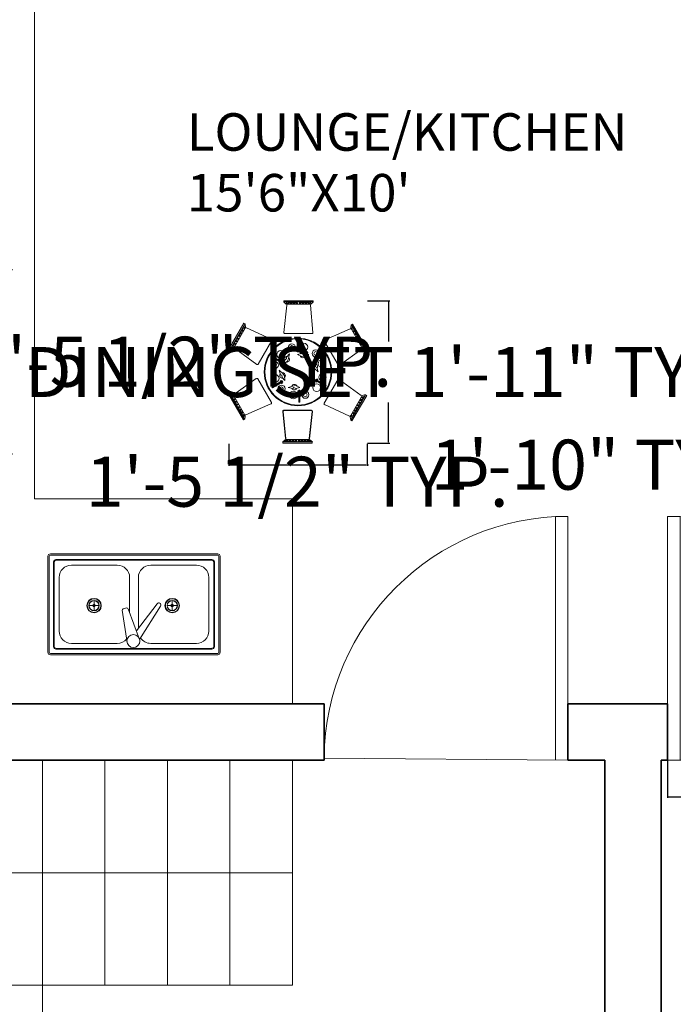
# Model space of a CAD drawing. Units: inches. Extents: x 125 to 976, y 231 to 853.
# Tile 3 of 16: x 219 to 324, y 455 to 613. Entities that reach past the tile are written whole.
import ezdxf

# ---------------------------------------------------------------- set-up
doc = ezdxf.new("R2010")
doc.units = ezdxf.units.IN
doc.header["$MEASUREMENT"] = 0
for name, color, linetype, lineweight in [('A-ANNO-DIMS', 2, 'Continuous', 18), ('A-AREA-IDEN', 7, 'Continuous', 18), ('A-DOOR', 3, 'Continuous', 18), ('A-FLOR-CASE', 32, 'Continuous', 18), ('A-FLOR-FIXT', 9, 'Continuous', 18), ('A-FLOR-STRS', 7, 'Continuous', 18), ('A-WALL', 7, 'Continuous', 35), ('Furniture', 8, 'Continuous', 15)]:
    doc.layers.add(name, color=color, linetype=linetype, lineweight=lineweight)
doc.styles.get("Standard").update_dxf_attribs({"font": 'italic8.shx'})
doc.dimstyles.get("Standard").update_dxf_attribs({"dimtxt": 8, "dimasz": 0.18, "dimexe": 0.18, "dimexo": 0.0625, "dimgap": 0.09, "dimtad": 0, "dimtih": 1, "dimtoh": 1, "dimdec": 4, "dimzin": 0, "dimdsep": 46, "dimlunit": 3, "dimtxsty": 'Standard', "dimcen": 0.09, "dimclrt": 4, "dimadec": 0, "dimazin": 0, "dimtfac": 1, "dimtdec": 4, "dimtofl": 0, "dimtmove": 0, "dimatfit": 3, "dimfxl": 1, "dimtolj": 1, "dimtzin": 0, "dimarcsym": 0})

# ---------------------------------------------------------------- blocks, each defined once
blk = doc.blocks.new('DINING-SET-ROUND-6')
for p, q in [((8.8, 22.58), (9.2, 22.26)), ((8.82, 17.72), (9.3, 22.08)), ((8.83, 22.8), (8.83, 22.6)), ((13.52, 22.8), (8.83, 22.8)), ((8.83, 22.6), (13.52, 22.6)), ((9.19, 22.53), (9.57, 22.55)), ((9.54, 22.27), (9.19, 22.53)), ((9.2, 22.26), (9.54, 22.27)), ((9.46, 22.23), (12.91, 22.23)), ((9.57, 22.55), (9.56, 22.32)), ((9.67, 22.56), (9.91, 22.32)), ((9.8, 22.55), (9.89, 22.55)), ((10.04, 22.32), (9.8, 22.55)), ((9.89, 22.55), (10.01, 22.45)), ((9.91, 22.32), (10.04, 22.32)), ((10.01, 22.45), (10.04, 22.48)), ((10.04, 22.48), (10.05, 22.34)), ((10.15, 22.56), (10.39, 22.32)), ((10.28, 22.55), (10.37, 22.55)), ((10.52, 22.32), (10.28, 22.55)), ((10.37, 22.55), (10.49, 22.45)), ((10.39, 22.32), (10.52, 22.32)), ((10.49, 22.45), (10.52, 22.48)), ((10.52, 22.48), (10.54, 22.34)), ((10.63, 22.56), (10.87, 22.32)), ((10.76, 22.55), (10.86, 22.55)), ((11, 22.32), (10.76, 22.55)), ((10.86, 22.55), (10.97, 22.45)), ((10.87, 22.32), (11, 22.32)), ((10.97, 22.45), (11, 22.48)), ((11, 22.48), (11.02, 22.34)), ((11.32, 22.48), (11.31, 22.34)), ((11.32, 22.32), (11.56, 22.55)), ((11.35, 22.45), (11.32, 22.48)), ((11.45, 22.32), (11.32, 22.32)), ((11.47, 22.55), (11.35, 22.45)), ((11.69, 22.56), (11.45, 22.32)), ((11.56, 22.55), (11.47, 22.55)), ((11.8, 22.48), (11.79, 22.34)), ((11.8, 22.32), (12.04, 22.55)), ((11.83, 22.45), (11.8, 22.48)), ((11.93, 22.32), (11.8, 22.32)), ((11.95, 22.55), (11.83, 22.45)), ((12.17, 22.56), (11.93, 22.32)), ((12.04, 22.55), (11.95, 22.55)), ((12.28, 22.48), (12.27, 22.34)), ((12.28, 22.32), (12.52, 22.55)), ((12.32, 22.45), (12.28, 22.48)), ((12.41, 22.32), (12.28, 22.32)), ((12.43, 22.55), (12.32, 22.45)), ((12.65, 22.56), (12.41, 22.32)), ((12.52, 22.55), (12.43, 22.55)), ((12.75, 22.55), (12.77, 22.32)), ((13.13, 22.53), (12.75, 22.55)), ((12.78, 22.27), (13.13, 22.53)), ((13.12, 22.26), (12.78, 22.27)), ((13.07, 22.08), (13.49, 17.72)), ((13.52, 22.58), (13.12, 22.26)), ((13.52, 22.6), (13.52, 22.8)), ((2.44, 19.22), (0.09, 15.16)), ((0.27, 15.05), (2.62, 19.11)), ((2.62, 19.11), (2.44, 19.22)), ((2.63, 19.1), (2.71, 18.6)), ((19.62, 18.97), (19.54, 18.47)), ((19.83, 19.06), (19.65, 18.95)), ((19.65, 18.95), (21.99, 14.9)), ((22.17, 15), (19.83, 19.06)), ((0.91, 15.41), (2.63, 18.4)), ((1.68, 17.39), (1.63, 17.31)), ((1.75, 17.07), (1.68, 17.39)), ((1.73, 17.51), (1.82, 17.18)), ((1.9, 17.58), (1.86, 17.57)), ((1.86, 17.57), (1.97, 17.48)), ((1.92, 17.81), (1.87, 17.73)), ((1.87, 17.73), (1.9, 17.58)), ((1.99, 17.49), (1.92, 17.81)), ((1.97, 17.93), (2.06, 17.6)), ((2.06, 17.6), (1.99, 17.49)), ((2.14, 18), (2.1, 17.99)), ((2.1, 17.99), (2.21, 17.9)), ((2.16, 18.23), (2.11, 18.14)), ((2.11, 18.14), (2.14, 18)), ((2.24, 17.91), (2.16, 18.23)), ((2.21, 18.35), (2.3, 18.02)), ((2.3, 18.02), (2.24, 17.91)), ((2.48, 18.75), (2.27, 18.42)), ((2.27, 18.42), (2.48, 18.32)), ((2.53, 18.31), (2.48, 18.75)), ((2.71, 18.6), (2.53, 18.31)), ((2.84, 18.46), (6.82, 16.65)), ((13.33, 17.54), (8.98, 17.54)), ((15.42, 16.53), (19.43, 18.29)), ((19.54, 18.47), (19.72, 18.18)), ((19.64, 18.23), (21.36, 15.24)), ((19.72, 18.18), (19.77, 18.62)), ((19.77, 18.62), (19.97, 18.29)), ((19.97, 18.29), (19.77, 18.19)), ((20.03, 18.21), (19.95, 17.89)), ((19.95, 17.89), (20.01, 17.77)), ((20.01, 17.77), (20.08, 18.1)), ((20.15, 17.86), (20.03, 17.77)), ((20.08, 18.1), (20.13, 18.01)), ((20.13, 18.01), (20.11, 17.87)), ((20.11, 17.87), (20.15, 17.86)), ((20.28, 17.8), (20.19, 17.47)), ((20.19, 17.47), (20.25, 17.36)), ((20.25, 17.36), (20.33, 17.68)), ((20.39, 17.44), (20.27, 17.35)), ((20.33, 17.68), (20.37, 17.6)), ((20.37, 17.6), (20.35, 17.45)), ((20.35, 17.45), (20.39, 17.44)), ((20.52, 17.38), (20.43, 17.05)), ((0.72, 15.76), (1.05, 15.85)), ((1.11, 15.96), (0.8, 15.86)), ((0.8, 15.86), (0.85, 15.95)), ((0.85, 15.95), (0.99, 16)), ((0.96, 16.18), (1.29, 16.27)), ((0.97, 16.04), (1.11, 15.98)), ((0.99, 16), (0.97, 16.04)), ((1.35, 16.38), (1.04, 16.28)), ((1.04, 16.28), (1.09, 16.36)), ((1.05, 15.85), (1.11, 15.96)), ((1.09, 16.36), (1.23, 16.41)), ((1.2, 16.59), (1.53, 16.68)), ((1.23, 16.41), (1.21, 16.46)), ((1.21, 16.46), (1.35, 16.4)), ((1.59, 16.79), (1.28, 16.7)), ((1.28, 16.7), (1.33, 16.78)), ((1.29, 16.27), (1.35, 16.38)), ((1.33, 16.78), (1.47, 16.83)), ((1.45, 16.87), (1.59, 16.82)), ((1.47, 16.83), (1.45, 16.87)), ((1.53, 16.68), (1.59, 16.79)), ((1.66, 17.16), (1.62, 17.15)), ((1.62, 17.15), (1.73, 17.07)), ((1.63, 17.31), (1.66, 17.16)), ((1.82, 17.18), (1.75, 17.07)), ((6.9, 16.42), (4.72, 12.66)), ((10.97, 16.52, 0.91), (10.97, 14.61, 0.91)), ((11.03, 16.52, 0.91), (10.97, 16.52, 0.91)), ((11.03, 14.61, 0.91), (11.03, 16.52, 0.91)), ((11.08, 16.52, 0.91), (11.08, 14.61, 0.91)), ((11.14, 16.52, 0.91), (11.08, 16.52, 0.91)), ((11.14, 14.61, 0.91), (11.14, 16.52, 0.91)), ((17.52, 12.54), (15.34, 16.3)), ((20.43, 17.05), (20.49, 16.94)), ((20.49, 16.94), (20.57, 17.26)), ((20.63, 17.02), (20.51, 16.94)), ((20.57, 17.26), (20.61, 17.18)), ((20.61, 17.18), (20.59, 17.03)), ((20.59, 17.03), (20.63, 17.02)), ((20.65, 16.66), (20.97, 16.57)), ((20.72, 16.55), (20.65, 16.66)), ((20.79, 16.74), (20.66, 16.69)), ((21.05, 16.46), (20.72, 16.55)), ((20.78, 16.7), (20.79, 16.74)), ((20.92, 16.65), (20.78, 16.7)), ((20.89, 16.25), (21.21, 16.15)), ((20.96, 16.14), (20.89, 16.25)), ((21.03, 16.33), (20.9, 16.27)), ((20.97, 16.57), (20.92, 16.65)), ((21.29, 16.05), (20.96, 16.14)), ((21.02, 16.28), (21.03, 16.33)), ((21.16, 16.23), (21.02, 16.28)), ((21.13, 15.83), (21.45, 15.73)), ((21.2, 15.72), (21.13, 15.83)), ((21.27, 15.91), (21.14, 15.85)), ((21.21, 16.15), (21.16, 16.23)), ((21.26, 15.87), (21.27, 15.91)), ((21.4, 15.82), (21.26, 15.87)), ((21.45, 15.73), (21.4, 15.82)), ((0.09, 15.16), (0.27, 15.05)), ((0.27, 15.02), (0.75, 15.21)), ((0.51, 15.33), (0.69, 15.67)), ((0.91, 15.51), (0.51, 15.33)), ((0.69, 15.67), (0.87, 15.54)), ((0.75, 15.21), (0.91, 15.51)), ((4.49, 12.61), (0.95, 15.2)), ((9.74, 14.31, 0.91), (9.23, 13.78, 0.91)), ((9.58, 13.56, 0.91), (9.74, 14.31, 0.91)), ((10.81, 14.88, 0.91), (10.81, 14.72, 0.91)), ((10.97, 14.88, 0.91), (10.81, 14.88, 0.91)), ((10.81, 14.72, 0.91), (10.97, 14.72, 0.91)), ((10.97, 14.61, 0.91), (11.03, 14.61, 0.91)), ((11.61, 14.37, 0.91), (10.99, 14.19, 0.91)), ((10.99, 14.19, 0.91), (11.68, 13.89, 0.91)), ((11.08, 14.88, 0.91), (11.03, 14.88, 0.91)), ((11.03, 14.72, 0.91), (11.08, 14.72, 0.91)), ((11.08, 14.61, 0.91), (11.14, 14.61, 0.91)), ((11.31, 14.88, 0.91), (11.14, 14.88, 0.91)), ((11.14, 14.72, 0.91), (11.31, 14.72, 0.91)), ((11.31, 14.72, 0.91), (11.31, 14.88, 0.91)), ((11.94, 14.21, 0.91), (11.61, 14.37, 0.91)), ((12.14, 14.36, 0.91), (11.94, 14.21, 0.91)), ((12.12, 13.95, 0.91), (12.85, 14.19, 0.91)), ((12.85, 14.19, 0.91), (12.14, 14.36, 0.91)), ((15.38, 14.23, 0.91), (13.72, 13.27, 0.91)), ((13.75, 13.22, 0.91), (15.41, 14.18, 0.91)), ((15.41, 14.18, 0.91), (15.38, 14.23, 0.91)), ((21.32, 15.03), (17.75, 12.49)), ((21.53, 15.63), (21.2, 15.72)), ((21.34, 15.37), (21.74, 15.2)), ((21.5, 15.07), (21.34, 15.37)), ((21.56, 15.54), (21.37, 15.41)), ((21.97, 14.89), (21.5, 15.07)), ((21.74, 15.2), (21.56, 15.54)), ((21.99, 14.9), (22.17, 15)), ((6.8, 13.9, 0.91), (6.77, 13.85, 0.91)), ((6.77, 13.85, 0.91), (8.43, 12.89, 0.91)), ((8.46, 12.94, 0.91), (6.8, 13.9, 0.91)), ((6.86, 14, 0.91), (6.83, 13.95, 0.91)), ((6.83, 13.95, 0.91), (8.49, 12.99, 0.91)), ((8.52, 13.04, 0.91), (6.86, 14, 0.91)), ((8.2, 13.02, 0.91), (8.12, 12.89, 0.91)), ((8.12, 12.89, 0.91), (8.26, 12.81, 0.91)), ((8.26, 13.12, 0.91), (8.23, 13.07, 0.91)), ((8.26, 12.81, 0.91), (8.34, 12.95, 0.91)), ((8.37, 13.32, 0.91), (8.29, 13.17, 0.91)), ((8.51, 13.24, 0.91), (8.37, 13.32, 0.91)), ((8.37, 13, 0.91), (8.39, 13.04, 0.91)), ((8.42, 13.1, 0.91), (8.51, 13.24, 0.91)), ((8.43, 12.89, 0.91), (8.46, 12.94, 0.91)), ((8.49, 12.99, 0.91), (8.52, 13.04, 0.91)), ((8.96, 13.32, 0.91), (8.81, 12.7, 0.91)), ((8.81, 12.7, 0.91), (9.41, 13.15, 0.91)), ((9.27, 13.54, 0.91), (8.96, 13.32, 0.91)), ((9.23, 13.78, 0.91), (9.27, 13.54, 0.91)), ((9.41, 13.15, 0.91), (9.58, 13.56, 0.91)), ((11.68, 13.89, 0.91), (12.12, 13.95, 0.91)), ((13.84, 12.59, 0.91), (13.37, 13.04, 0.91)), ((13.37, 13.04, 0.91), (13.46, 12.29, 0.91)), ((13.72, 13.27, 0.91), (13.75, 13.22, 0.91)), ((13.88, 13.54, 0.91), (13.74, 13.46, 0.91)), ((13.74, 13.46, 0.91), (13.82, 13.33, 0.91)), ((15.44, 14.13, 0.91), (13.78, 13.17, 0.91)), ((13.78, 13.17, 0.91), (13.81, 13.12, 0.91)), ((13.81, 13.12, 0.91), (15.47, 14.08, 0.91)), ((13.85, 13.27, 0.91), (13.88, 13.23, 0.91)), ((13.96, 13.4, 0.91), (13.88, 13.54, 0.91)), ((13.91, 13.18, 0.91), (13.99, 13.03, 0.91)), ((14.01, 13.31, 0.91), (13.99, 13.35, 0.91)), ((13.99, 13.03, 0.91), (14.13, 13.11, 0.91)), ((14.13, 13.11, 0.91), (14.04, 13.25, 0.91)), ((15.47, 14.08, 0.91), (15.44, 14.13, 0.91)), ((8.08, 11.67, 0.91), (8.28, 10.97, 0.91)), ((8.64, 11.17, 0.91), (8.08, 11.67, 0.91)), ((8.92, 10.81, 0.91), (8.64, 11.17, 0.91)), ((13.46, 12.29, 0.91), (13.73, 11.94, 0.91)), ((13.73, 11.94, 0.91), (14.3, 11.43, 0.91)), ((13.87, 12.23, 0.91), (13.84, 12.59, 0.91)), ((14.09, 12.13, 0.91), (13.87, 12.23, 0.91)), ((14.3, 11.43, 0.91), (14.09, 12.13, 0.91)), ((0.85, 7.79), (4.42, 10.34)), ((4.65, 10.29), (6.83, 6.52)), ((8.57, 9.99, 0.91), (6.91, 9.03, 0.91)), ((6.94, 8.97, 0.91), (8.6, 9.93, 0.91)), ((8.62, 9.89, 0.91), (6.96, 8.93, 0.91)), ((6.99, 8.88, 0.91), (8.65, 9.84, 0.91)), ((8.38, 10.07, 0.91), (8.25, 10, 0.91)), ((8.25, 10, 0.91), (8.33, 9.85, 0.91)), ((8.28, 10.97, 0.91), (8.51, 10.88, 0.91)), ((8.36, 9.8, 0.91), (8.39, 9.75, 0.91)), ((8.47, 9.93, 0.91), (8.38, 10.07, 0.91)), ((8.42, 9.7, 0.91), (8.5, 9.57, 0.91)), ((8.53, 9.83, 0.91), (8.5, 9.88, 0.91)), ((8.5, 9.57, 0.91), (8.63, 9.64, 0.91)), ((8.51, 10.88, 0.91), (8.54, 10.51, 0.91)), ((8.54, 10.51, 0.91), (9, 10.06, 0.91)), ((8.63, 9.64, 0.91), (8.56, 9.78, 0.91)), ((8.6, 9.93, 0.91), (8.57, 9.99, 0.91)), ((8.65, 9.84, 0.91), (8.62, 9.89, 0.91)), ((9, 10.06, 0.91), (8.92, 10.81, 0.91)), ((12.79, 9.54, 0.91), (12.64, 8.8, 0.91)), ((12.96, 9.95, 0.91), (12.79, 9.54, 0.91)), ((13.57, 10.41, 0.91), (12.96, 9.95, 0.91)), ((13.11, 9.57, 0.91), (13.41, 9.78, 0.91)), ((13.14, 9.33, 0.91), (13.11, 9.57, 0.91)), ((13.41, 9.78, 0.91), (13.57, 10.41, 0.91)), ((13.88, 10.12, 0.91), (13.85, 10.07, 0.91)), ((13.85, 10.07, 0.91), (15.52, 9.11, 0.91)), ((13.95, 10.01, 0.91), (13.87, 9.86, 0.91)), ((13.87, 9.86, 0.91), (14, 9.79, 0.91)), ((15.55, 9.16, 0.91), (13.88, 10.12, 0.91)), ((13.94, 10.22, 0.91), (13.91, 10.17, 0.91)), ((13.91, 10.17, 0.91), (15.57, 9.21, 0.91)), ((15.6, 9.26, 0.91), (13.94, 10.22, 0.91)), ((14.01, 10.11, 0.91), (13.98, 10.06, 0.91)), ((14, 9.79, 0.91), (14.09, 9.93, 0.91)), ((14.12, 10.3, 0.91), (14.04, 10.16, 0.91)), ((14.25, 10.22, 0.91), (14.12, 10.3, 0.91)), ((14.12, 9.98, 0.91), (14.15, 10.03, 0.91)), ((14.18, 10.08, 0.91), (14.25, 10.22, 0.91)), ((15.28, 6.4), (17.45, 10.17)), ((17.68, 10.22), (21.22, 7.62)), ((0.18, 7.93), (0, 7.82)), ((2.53, 3.87), (0.18, 7.93)), ((0.2, 7.94), (0.68, 7.75)), ((6.91, 9.03, 0.91), (6.94, 8.97, 0.91)), ((6.96, 8.93, 0.91), (6.99, 8.88, 0.91)), ((10.25, 9.16, 0.91), (9.53, 8.92, 0.91)), ((9.53, 8.92, 0.91), (10.24, 8.75, 0.91)), ((10.24, 8.75, 0.91), (10.43, 8.9, 0.91)), ((10.69, 9.22, 0.91), (10.25, 9.16, 0.91)), ((10.43, 8.9, 0.91), (10.77, 8.74, 0.91)), ((11.39, 8.92, 0.91), (10.69, 9.22, 0.91)), ((10.77, 8.74, 0.91), (11.39, 8.92, 0.91)), ((11.23, 8.39, 0.91), (11.07, 8.39, 0.91)), ((11.07, 8.39, 0.91), (11.07, 8.23, 0.91)), ((11.07, 8.23, 0.91), (11.23, 8.23, 0.91)), ((11.29, 8.5, 0.91), (11.23, 8.5, 0.91)), ((11.23, 8.5, 0.91), (11.23, 6.58, 0.91)), ((11.29, 6.58, 0.91), (11.29, 8.5, 0.91)), ((11.35, 8.39, 0.91), (11.29, 8.39, 0.91)), ((11.29, 8.23, 0.91), (11.35, 8.23, 0.91)), ((11.41, 8.5, 0.91), (11.35, 8.5, 0.91)), ((11.35, 8.5, 0.91), (11.35, 6.58, 0.91)), ((11.41, 6.58, 0.91), (11.41, 8.5, 0.91)), ((11.56, 8.39, 0.91), (11.41, 8.39, 0.91)), ((11.41, 8.23, 0.91), (11.56, 8.23, 0.91)), ((11.56, 8.23, 0.91), (11.56, 8.39, 0.91)), ((12.64, 8.8, 0.91), (13.14, 9.33, 0.91)), ((15.52, 9.11, 0.91), (15.55, 9.16, 0.91)), ((15.57, 9.21, 0.91), (15.6, 9.26, 0.91)), ((0, 7.82), (2.35, 3.77)), ((0.43, 7.63), (0.61, 7.29)), ((0.83, 7.45), (0.43, 7.63)), ((0.61, 7.29), (0.8, 7.41)), ((0.64, 7.19), (0.97, 7.11)), ((0.68, 7.75), (0.83, 7.45)), ((0.72, 7.09), (0.77, 7.01)), ((1.04, 6.99), (0.72, 7.09)), ((0.77, 7.01), (0.91, 6.96)), ((2.53, 4.6), (0.81, 7.58)), ((0.88, 6.78), (1.21, 6.69)), ((0.9, 6.91), (1.03, 6.97)), ((0.91, 6.96), (0.9, 6.91)), ((0.96, 6.67), (1.01, 6.59)), ((1.28, 6.58), (0.96, 6.67)), ((0.97, 7.11), (1.04, 6.99)), ((1.01, 6.59), (1.15, 6.54)), ((1.13, 6.36), (1.45, 6.27)), ((1.14, 6.5), (1.27, 6.56)), ((1.15, 6.54), (1.14, 6.5)), ((1.21, 6.69), (1.28, 6.58)), ((11.23, 6.58, 0.91), (11.29, 6.58, 0.91)), ((11.35, 6.58, 0.91), (11.41, 6.58, 0.91)), ((21.26, 7.41), (19.54, 4.43)), ((21.9, 7.77), (19.55, 3.71)), ((19.73, 3.61), (22.08, 7.67)), ((20.88, 6.56), (20.82, 6.45)), ((20.82, 6.45), (21.13, 6.54)), ((20.96, 6.37), (20.82, 6.43)), ((21.21, 6.65), (20.88, 6.56)), ((21.08, 6.46), (20.94, 6.41)), ((20.94, 6.41), (20.96, 6.37)), ((21.12, 6.98), (21.06, 6.86)), ((21.06, 6.86), (21.37, 6.96)), ((21.2, 6.78), (21.06, 6.84)), ((21.13, 6.54), (21.08, 6.46)), ((21.45, 7.06), (21.12, 6.98)), ((21.33, 6.88), (21.19, 6.83)), ((21.19, 6.83), (21.2, 6.78)), ((21.42, 7.62), (21.27, 7.32)), ((21.27, 7.32), (21.66, 7.5)), ((21.49, 7.15), (21.3, 7.28)), ((21.37, 6.96), (21.33, 6.88)), ((21.9, 7.81), (21.42, 7.62)), ((21.66, 7.5), (21.49, 7.15)), ((22.08, 7.67), (21.9, 7.77)), ((1.2, 6.26), (1.25, 6.17)), ((1.52, 6.16), (1.2, 6.26)), ((1.25, 6.17), (1.39, 6.12)), ((1.38, 6.08), (1.51, 6.14)), ((1.39, 6.12), (1.38, 6.08)), ((1.45, 6.27), (1.52, 6.16)), ((1.54, 5.8), (1.66, 5.89)), ((1.58, 5.79), (1.54, 5.8)), ((1.56, 5.65), (1.58, 5.79)), ((1.6, 5.56), (1.56, 5.65)), ((1.68, 5.88), (1.6, 5.56)), ((1.65, 5.44), (1.74, 5.77)), ((1.74, 5.77), (1.68, 5.88)), ((1.78, 5.39), (1.9, 5.47)), ((1.82, 5.37), (1.78, 5.39)), ((1.8, 5.23), (1.82, 5.37)), ((1.85, 5.15), (1.8, 5.23)), ((1.92, 5.47), (1.85, 5.15)), ((1.9, 5.03), (1.98, 5.35)), ((1.98, 5.35), (1.92, 5.47)), ((2.02, 4.97), (2.14, 5.06)), ((2.07, 4.96), (2.02, 4.97)), ((2.04, 4.81), (2.07, 4.96)), ((2.09, 4.73), (2.04, 4.81)), ((2.16, 5.05), (2.09, 4.73)), ((2.14, 4.61), (2.22, 4.94)), ((2.22, 4.94), (2.16, 5.05)), ((6.75, 6.3), (2.74, 4.53)), ((9.1, 0.74), (8.68, 5.1)), ((9.14, 0.73), (8.73, 5.09)), ((8.84, 5.28), (13.19, 5.28)), ((8.89, 5.26), (13.23, 5.26)), ((13.35, 5.1), (12.87, 0.74)), ((13.39, 5.09), (12.91, 0.72)), ((19.33, 4.36), (15.35, 6.18)), ((19.87, 4.81), (19.94, 4.92)), ((19.96, 4.48), (19.87, 4.81)), ((19.94, 4.92), (20.01, 4.6)), ((20.07, 4.84), (19.96, 4.92)), ((20.03, 4.83), (20.07, 4.84)), ((20.06, 4.68), (20.03, 4.83)), ((20.11, 5.22), (20.18, 5.34)), ((20.2, 4.9), (20.11, 5.22)), ((20.18, 5.34), (20.25, 5.01)), ((20.31, 5.26), (20.2, 5.34)), ((20.25, 5.01), (20.3, 5.1)), ((20.27, 5.24), (20.31, 5.26)), ((20.3, 5.1), (20.27, 5.24)), ((20.35, 5.64), (20.42, 5.75)), ((20.44, 5.31), (20.35, 5.64)), ((20.42, 5.75), (20.49, 5.43)), ((20.56, 5.67), (20.44, 5.76)), ((20.49, 5.43), (20.54, 5.51)), ((20.51, 5.66), (20.56, 5.67)), ((20.54, 5.51), (20.51, 5.66)), ((20.64, 6.14), (20.58, 6.03)), ((20.58, 6.03), (20.89, 6.13)), ((20.72, 5.95), (20.58, 6.01)), ((20.97, 6.23), (20.64, 6.14)), ((20.84, 6.04), (20.7, 5.99)), ((20.7, 5.99), (20.72, 5.95)), ((20.89, 6.13), (20.84, 6.04)), ((2.2, 4.53), (2.4, 4.63)), ((2.4, 4.21), (2.2, 4.53)), ((2.35, 3.77), (2.53, 3.87)), ((2.45, 4.64), (2.4, 4.21)), ((2.63, 4.36), (2.45, 4.64)), ((2.56, 3.85), (2.63, 4.36)), ((19.46, 4.23), (19.64, 4.51)), ((19.54, 3.72), (19.46, 4.23)), ((19.55, 3.71), (19.73, 3.61)), ((19.64, 4.51), (19.69, 4.08)), ((19.9, 4.4), (19.69, 4.5)), ((19.69, 4.08), (19.9, 4.4)), ((20.01, 4.6), (20.06, 4.68)), ((8.65, 0.24), (9.05, 0.57)), ((8.65, 0.23), (8.65, 0.02)), ((13.34, 0.23), (8.65, 0.23)), ((8.65, 0.02), (13.34, 0.02)), ((8.69, 0.23), (9.09, 0.55)), ((8.69, 0.21), (8.69, 0)), ((13.38, 0.21), (8.69, 0.21)), ((8.69, 0), (13.38, 0)), ((9.39, 0.55), (9.04, 0.29)), ((9.04, 0.29), (9.42, 0.28)), ((9.05, 0.57), (9.39, 0.55)), ((9.43, 0.53), (9.08, 0.28)), ((9.08, 0.28), (9.46, 0.26)), ((9.09, 0.55), (9.43, 0.53)), ((12.71, 0.6), (9.26, 0.6)), ((12.75, 0.58), (9.3, 0.58)), ((9.42, 0.28), (9.41, 0.5)), ((9.46, 0.26), (9.45, 0.49)), ((9.52, 0.26), (9.76, 0.5)), ((9.56, 0.25), (9.8, 0.49)), ((9.89, 0.5), (9.65, 0.28)), ((9.65, 0.28), (9.74, 0.28)), ((9.93, 0.49), (9.69, 0.26)), ((9.69, 0.26), (9.78, 0.26)), ((9.74, 0.28), (9.85, 0.37)), ((9.76, 0.5), (9.89, 0.5)), ((9.78, 0.26), (9.9, 0.36)), ((9.8, 0.49), (9.93, 0.49)), ((9.85, 0.37), (9.89, 0.34)), ((9.89, 0.34), (9.9, 0.49)), ((9.9, 0.36), (9.93, 0.33)), ((9.93, 0.33), (9.94, 0.47)), ((10, 0.26), (10.24, 0.5)), ((10.04, 0.25), (10.28, 0.49)), ((10.37, 0.5), (10.13, 0.28)), ((10.13, 0.28), (10.22, 0.28)), ((10.41, 0.49), (10.17, 0.26)), ((10.17, 0.26), (10.27, 0.26)), ((10.22, 0.28), (10.34, 0.37)), ((10.24, 0.5), (10.37, 0.5)), ((10.27, 0.26), (10.38, 0.36)), ((10.28, 0.49), (10.41, 0.49)), ((10.34, 0.37), (10.37, 0.34)), ((10.37, 0.34), (10.38, 0.49)), ((10.38, 0.36), (10.41, 0.33)), ((10.41, 0.33), (10.43, 0.47)), ((10.48, 0.26), (10.72, 0.5)), ((10.52, 0.25), (10.76, 0.49)), ((10.85, 0.5), (10.61, 0.28)), ((10.61, 0.28), (10.71, 0.28)), ((10.89, 0.49), (10.65, 0.26)), ((10.65, 0.26), (10.75, 0.26)), ((10.71, 0.28), (10.82, 0.37)), ((10.72, 0.5), (10.85, 0.5)), ((10.75, 0.26), (10.86, 0.36)), ((10.76, 0.49), (10.89, 0.49)), ((10.82, 0.37), (10.85, 0.34)), ((10.85, 0.34), (10.87, 0.49)), ((10.86, 0.36), (10.89, 0.33)), ((10.89, 0.33), (10.91, 0.47)), ((11.17, 0.34), (11.15, 0.49)), ((11.17, 0.5), (11.41, 0.28)), ((11.3, 0.5), (11.17, 0.5)), ((11.2, 0.37), (11.17, 0.34)), ((11.21, 0.33), (11.2, 0.47)), ((11.31, 0.28), (11.2, 0.37)), ((11.21, 0.49), (11.45, 0.26)), ((11.34, 0.49), (11.21, 0.49)), ((11.24, 0.36), (11.21, 0.33)), ((11.36, 0.26), (11.24, 0.36)), ((11.54, 0.26), (11.3, 0.5)), ((11.41, 0.28), (11.31, 0.28)), ((11.58, 0.25), (11.34, 0.49)), ((11.45, 0.26), (11.36, 0.26)), ((11.65, 0.34), (11.64, 0.49)), ((11.65, 0.5), (11.89, 0.28)), ((11.78, 0.5), (11.65, 0.5)), ((11.68, 0.37), (11.65, 0.34)), ((11.69, 0.33), (11.68, 0.47)), ((11.8, 0.28), (11.68, 0.37)), ((11.69, 0.49), (11.93, 0.26)), ((11.82, 0.49), (11.69, 0.49)), ((11.73, 0.36), (11.69, 0.33)), ((11.84, 0.26), (11.73, 0.36)), ((12.02, 0.26), (11.78, 0.5)), ((11.89, 0.28), (11.8, 0.28)), ((12.06, 0.25), (11.82, 0.49)), ((11.93, 0.26), (11.84, 0.26)), ((12.13, 0.34), (12.12, 0.49)), ((12.13, 0.5), (12.37, 0.28)), ((12.26, 0.5), (12.13, 0.5)), ((12.17, 0.37), (12.13, 0.34)), ((12.17, 0.33), (12.16, 0.47)), ((12.17, 0.49), (12.42, 0.26)), ((12.3, 0.49), (12.17, 0.49)), ((12.28, 0.28), (12.17, 0.37)), ((12.21, 0.36), (12.17, 0.33)), ((12.32, 0.26), (12.21, 0.36)), ((12.5, 0.26), (12.26, 0.5)), ((12.37, 0.28), (12.28, 0.28)), ((12.54, 0.25), (12.3, 0.49)), ((12.42, 0.26), (12.32, 0.26)), ((12.6, 0.28), (12.61, 0.5)), ((12.98, 0.29), (12.6, 0.28)), ((12.97, 0.57), (12.63, 0.55)), ((12.63, 0.55), (12.98, 0.29)), ((12.64, 0.26), (12.66, 0.49)), ((13.02, 0.28), (12.64, 0.26)), ((13.01, 0.55), (12.67, 0.53)), ((12.67, 0.53), (13.02, 0.28)), ((13.37, 0.24), (12.97, 0.57)), ((13.41, 0.23), (13.01, 0.55)), ((13.34, 0.02), (13.34, 0.23)), ((13.38, 0), (13.38, 0.21))]:
    blk.add_line(p, q)
for centre, radius in [((11.09, 11.41), 5.4), ((11.09, 11.41), 5.3), ((10.11, 15.33, 0.91), 0.572), ((12.04, 15.38, 0.91), 0.616), ((8.3, 14.2, 0.91), 0.616), ((10.13, 15.34, 0.91), 0.295), ((13.92, 14.37, 0.91), 0.572), ((13.94, 14.37, 0.91), 0.295), ((7.38, 12.51, 0.91), 0.572), ((7.38, 12.53, 0.91), 0.295), ((14.93, 12.73, 0.91), 0.616), ((15, 10.59, 0.91), 0.572), ((7.45, 10.38, 0.91), 0.616), ((14.08, 8.9, 0.91), 0.616), ((15, 10.58, 0.91), 0.295), ((8.45, 8.73, 0.91), 0.572), ((8.44, 8.74, 0.91), 0.295), ((10.34, 7.73, 0.91), 0.616), ((12.26, 7.77, 0.91), 0.572), ((12.25, 7.77, 0.91), 0.295)]:
    blk.add_circle(centre, radius)
for centre, radius, start, end in [((9.46, 22.07), 0.16, 90, 173.7428), ((12.91, 22.07), 0.16, 5.4801, 90), ((2.77, 18.32), 0.16, 65.4801, 150), ((8.98, 17.7), 0.16, 173.7428, 270), ((13.33, 17.7), 0.16, 270, 5.4801), ((19.5, 18.15), 0.16, 30, 113.7428), ((6.76, 16.5), 0.16, 330, 65.4801), ((15.48, 16.38), 0.16, 113.7428, 210), ((1.05, 15.33), 0.16, 150, 233.7428), ((11.86, 14.13, 0.91), 0.448, 26.6641, 154.1442), ((21.22, 15.16), 0.16, 305.4801, 30), ((4.58, 12.74), 0.16, 233.7428, 330), ((9.3, 13.42, 0.91), 0.448, 86.6641, 214.1442), ((9.3, 13.42, 0.91), 0.448, 257.0611, 44.0662), ((11.86, 14.13, 0.91), 0.448, 197.0611, 344.0662), ((13.76, 12.26, 0.91), 0.448, 326.6641, 94.1442), ((8.62, 10.85, 0.91), 0.448, 146.6641, 274.1442), ((8.62, 10.85, 0.91), 0.448, 317.0611, 104.0662), ((13.76, 12.26, 0.91), 0.448, 137.0611, 284.0662), ((17.66, 12.62), 0.16, 210, 305.4801), ((4.52, 10.21), 0.16, 30, 125.4801), ((13.08, 9.68, 0.91), 0.448, 77.0611, 224.0662), ((13.08, 9.68, 0.91), 0.448, 266.6641, 34.1442), ((17.59, 10.09), 0.16, 53.7428, 150), ((10.51, 8.98, 0.91), 0.448, 17.0611, 164.0662), ((10.51, 8.98, 0.91), 0.448, 206.6641, 334.1442), ((0.95, 7.66), 0.16, 125.4801, 210), ((6.69, 6.44), 0.16, 293.7428, 30), ((15.41, 6.32), 0.16, 150, 245.4801), ((21.13, 7.49), 0.16, 330, 53.7428), ((8.84, 5.12), 0.16, 90, 185.4801), ((8.89, 5.1), 0.16, 90, 185.4801), ((13.19, 5.12), 0.16, 353.7428, 90), ((13.23, 5.1), 0.16, 353.7428, 90), ((2.67, 4.68), 0.16, 210, 293.7428), ((19.4, 4.51), 0.16, 245.4801, 330), ((9.26, 0.76), 0.16, 185.4801, 270), ((9.3, 0.74), 0.16, 185.4801, 270), ((12.71, 0.76), 0.16, 270, 353.7428), ((12.75, 0.74), 0.16, 270, 353.7428)]:
    blk.add_arc(centre, radius, start, end)
blk = doc.blocks.new('SINK-DOUBLE')
for p, q in [((27.17, 16.14), (0.4, 16.14)), ((27.17, 15.94), (0.4, 15.94)), ((0, 15.74), (0, 0.39)), ((0.2, 15.74), (0.2, 0.39)), ((0.91, 14.84), (0.91, 1.3)), ((1.03, 14.84), (1.03, 1.3)), ((26.26, 15.23), (1.3, 15.23)), ((26.26, 15.11), (1.3, 15.11)), ((11.11, 14.33), (3.78, 14.33)), ((23.78, 14.33), (16.46, 14.33)), ((26.54, 1.3), (26.54, 14.84)), ((26.66, 1.3), (26.66, 14.84)), ((27.37, 0.39), (27.37, 15.74)), ((27.56, 0.39), (27.56, 15.74)), ((1.81, 12.36), (1.81, 3.78)), ((13.07, 6.7), (13.07, 12.36)), ((14.49, 12.36), (14.49, 4.26)), ((25.75, 3.78), (25.75, 12.36)), ((7.39, 8.06), (7.39, 8.65)), ((14.16, 3.83), (17.49, 8.16)), ((17.92, 8.22), (17.95, 8.2)), ((19.9, 8.06), (19.9, 8.65)), ((7.18, 7.86), (6.59, 7.86)), ((7.39, 7.65), (7.39, 7.06)), ((7.59, 7.86), (8.18, 7.86)), ((11.9, 7.12), (12.69, 1.93)), ((12.59, 7.48), (12.04, 7.34)), ((14.68, 2.43), (12.83, 7.36)), ((14.68, 2.43), (18.03, 7.78)), ((19.7, 7.86), (19.11, 7.86)), ((19.9, 7.65), (19.9, 7.06)), ((20.11, 7.86), (20.7, 7.86)), ((3.78, 1.81), (11.11, 1.81)), ((16.46, 1.81), (23.78, 1.81)), ((0.4, 0.19), (27.17, 0.19)), ((1.3, 1.02), (26.26, 1.02)), ((1.3, 0.9), (26.26, 0.9)), ((0.4, 0), (27.17, 0))]:
    blk.add_line(p, q)
for centre, radius in [((7.39, 7.86), 1.16), ((7.39, 7.86), 1.1), ((7.39, 7.86), 0.83), ((7.39, 7.86), 0.794), ((7.39, 7.86), 0.204), ((7.39, 7.86), 0.0958), ((19.9, 7.86), 1.16), ((19.9, 7.86), 1.1), ((19.9, 7.86), 0.83), ((19.9, 7.86), 0.794), ((19.9, 7.86), 0.204), ((19.9, 7.86), 0.0958), ((13.69, 2.18), 1.03)]:
    blk.add_circle(centre, radius)
for centre, radius, start, end in [((0.4, 15.74), 0.394, 90, 180), ((0.4, 15.74), 0.197, 90, 180), ((27.17, 15.74), 0.394, 0, 90), ((27.17, 15.74), 0.197, 0, 90), ((1.3, 14.84), 0.394, 90, 180), ((1.3, 14.84), 0.276, 90, 180), ((3.78, 12.36), 1.97, 90, 180), ((11.11, 12.36), 1.97, 0, 90), ((16.46, 12.36), 1.97, 90, 180), ((23.78, 12.36), 1.97, 0, 90), ((26.26, 14.84), 0.394, 0, 90), ((26.26, 14.84), 0.276, 0, 90), ((17.74, 7.97), 0.315, 53.6309, 142.4185), ((17.76, 7.95), 0.315, 327.9301, 53.6309), ((12.09, 7.15), 0.197, 104.3233, 188.6985), ((12.64, 7.29), 0.197, 20.6498, 104.3233), ((3.78, 3.78), 1.97, 180, 270), ((23.78, 3.78), 1.97, 270, 0), ((11.11, 3.78), 1.97, 270, 319.575), ((16.46, 3.78), 1.97, 214.0864, 270), ((0.4, 0.39), 0.394, 180, 270), ((0.4, 0.39), 0.197, 180, 270), ((1.3, 1.3), 0.394, 180, 270), ((1.3, 1.3), 0.276, 180, 270), ((26.26, 1.3), 0.276, 270, 0), ((26.26, 1.3), 0.394, 270, 0), ((27.17, 0.39), 0.197, 270, 0), ((27.17, 0.39), 0.394, 270, 0)]:
    blk.add_arc(centre, radius, start, end)
blk = doc.blocks.new('DOOR-39IN-LH')
for p, q in [((-2, 0), (-2, 38.95)), ((0, 0), (0, 39)), ((-39, 0.34), (0, 0))]:
    blk.add_line(p, q)
blk.add_arc((0, 0), 39, 90, 179.5065)
blk = doc.blocks.new('DOOR-39IN-RH')
for p, q in [((0, 39), (0, 0)), ((2, 38.95), (2, 0)), ((0, 0), (39, 0))]:
    blk.add_line(p, q)
blk.add_arc((0, 0), 39, 0, 90)
blk = doc.blocks.new('*D40')
at = {"layer": 'A-ANNO-DIMS', "color": 0, "lineweight": -2, "transparency": 16777216}
for p, q in [((322.59, 494.04), (322.59, 488.07)), ((361.59, 494.04), (361.59, 488.07)), ((322.77, 488.25), (361.41, 488.25)), ((361.59, 488.25), (361.77, 488.25))]:
    blk.add_line(p, q, dxfattribs=at)
at = {"layer": 'A-ANNO-DIMS', "color": 0, "transparency": 16777216}
for points in [[(322.77, 488.28), (322.77, 488.22), (322.59, 488.25)], [(361.41, 488.28), (361.41, 488.22), (361.59, 488.25)]]:
    blk.add_solid(points, dxfattribs=at)
at = {"layer": 'Defpoints', "color": 0, "transparency": 16777216}
for p in [(322.59, 494.1), (361.59, 494.1), (361.59, 488.25)]:
    blk.add_point(p, dxfattribs=at)
at = {"layer": 'A-ANNO-DIMS', "color": 4, "transparency": 16777216, "insert": (432.52, 488.25), "char_height": 8, "attachment_point": 5}
blk.add_mtext('\\A1;RH DOOR 3\'-3" TYP.', dxfattribs=at)
blk = doc.blocks.new('*D46')
at = {"layer": 'A-ANNO-DIMS', "color": 0, "lineweight": -2, "transparency": 16777216}
for p, q in [((274.61, 567.59), (278.15, 567.59)), ((277.97, 567.41), (277.97, 561.05)), ((277.97, 544.97), (277.97, 551.34)), ((274.61, 544.79), (278.15, 544.79))]:
    blk.add_line(p, q, dxfattribs=at)
at = {"layer": 'A-ANNO-DIMS', "color": 0, "transparency": 16777216}
for points in [[(277.94, 567.41), (278, 567.41), (277.97, 567.59)], [(277.94, 544.97), (278, 544.97), (277.97, 544.79)]]:
    blk.add_solid(points, dxfattribs=at)
at = {"layer": 'Defpoints', "color": 0, "transparency": 16777216}
for p in [(274.55, 567.59), (277.97, 567.59), (274.55, 544.79)]:
    blk.add_point(p, dxfattribs=at)
at = {"layer": 'A-ANNO-DIMS', "color": 4, "transparency": 16777216, "insert": (277.97, 556.19), "char_height": 8, "attachment_point": 5}
blk.add_mtext('\\A1;DINING SET 1\'-11" TYP.', dxfattribs=at)
blk = doc.blocks.new('*D47')
at = {"layer": 'A-ANNO-DIMS', "color": 0, "lineweight": -2, "transparency": 16777216}
for p, q in [((252.38, 544.73), (252.38, 541.19)), ((274.55, 544.73), (274.55, 541.19)), ((252.56, 541.37), (274.37, 541.37)), ((274.55, 541.37), (274.73, 541.37))]:
    blk.add_line(p, q, dxfattribs=at)
at = {"layer": 'A-ANNO-DIMS', "color": 0, "transparency": 16777216}
for points in [[(252.56, 541.4), (252.56, 541.34), (252.38, 541.37)], [(274.37, 541.4), (274.37, 541.34), (274.55, 541.37)]]:
    blk.add_solid(points, dxfattribs=at)
at = {"layer": 'Defpoints', "color": 0, "transparency": 16777216}
for p in [(252.38, 544.79), (274.55, 544.79), (274.55, 541.37)]:
    blk.add_point(p, dxfattribs=at)
at = {"layer": 'A-ANNO-DIMS', "color": 4, "transparency": 16777216, "insert": (312.15, 541.37), "char_height": 8, "attachment_point": 5}
blk.add_mtext('\\A1;1\'-10" TYP.', dxfattribs=at)
blk = doc.blocks.new('*D50')
at = {"layer": 'A-ANNO-DIMS', "color": 0, "lineweight": -2, "transparency": 16777216}
for p, q in [((213.24, 572.61), (217.79, 572.61)), ((217.61, 572.43), (217.61, 564.03)), ((217.61, 543.26), (217.61, 551.66)), ((213.24, 543.08), (217.79, 543.08))]:
    blk.add_line(p, q, dxfattribs=at)
at = {"layer": 'A-ANNO-DIMS', "color": 0, "transparency": 16777216}
for points in [[(217.58, 572.43), (217.64, 572.43), (217.61, 572.61)], [(217.58, 543.26), (217.64, 543.26), (217.61, 543.08)]]:
    blk.add_solid(points, dxfattribs=at)
at = {"layer": 'Defpoints', "color": 0, "transparency": 16777216}
for p in [(213.18, 572.61), (217.61, 572.61), (213.18, 543.08)]:
    blk.add_point(p, dxfattribs=at)
at = {"layer": 'A-ANNO-DIMS', "color": 4, "transparency": 16777216, "insert": (217.61, 557.84), "char_height": 8, "attachment_point": 5}
blk.add_mtext('\\A1;COOKTOP 2\'-5 1/2" TYP.', dxfattribs=at)
blk = doc.blocks.new('*D51')
at = {"layer": 'A-ANNO-DIMS', "color": 0, "lineweight": -2, "transparency": 16777216}
for p, q in [((195.85, 543.02), (195.85, 538.47)), ((213.18, 543.02), (213.18, 538.47)), ((196.03, 538.65), (213, 538.65)), ((213.18, 538.65), (213.36, 538.65))]:
    blk.add_line(p, q, dxfattribs=at)
at = {"layer": 'A-ANNO-DIMS', "color": 0, "transparency": 16777216}
for points in [[(196.03, 538.68), (196.03, 538.62), (195.85, 538.65)], [(213, 538.68), (213, 538.62), (213.18, 538.65)]]:
    blk.add_solid(points, dxfattribs=at)
at = {"layer": 'Defpoints', "color": 0, "transparency": 16777216}
for p in [(195.85, 543.08), (213.18, 543.08), (213.18, 538.65)]:
    blk.add_point(p, dxfattribs=at)
at = {"layer": 'A-ANNO-DIMS', "color": 4, "transparency": 16777216, "insert": (263.35, 538.65), "char_height": 8, "attachment_point": 5}
blk.add_mtext('\\A1;1\'-5 1/2" TYP.', dxfattribs=at)

msp = doc.modelspace()

# ---------------------------------------------------------------- linework, layer by layer
at = {"layer": 'A-FLOR-CASE'}
for p, q in [((221.33932, 535.92817), (221.33932, 614.10475)), ((262.5792, 535.92817), (221.33932, 535.92817)), ((262.5792, 535.92817), (262.5792, 503.10475))]:
    msp.add_line(p, q, dxfattribs=at)
at = {"layer": 'A-FLOR-STRS'}
for p, q in [((222.5792, 494.10475), (222.5792, 358.10475)), ((232.5792, 494.10475), (232.5792, 458.10475)), ((242.5792, 494.10475), (242.5792, 458.10475)), ((252.5792, 494.10475), (252.5792, 458.10475)), ((262.5792, 494.10475), (262.5792, 458.10475)), ((262.5792, 476.10475), (204.18906, 476.10475)), ((262.5792, 458.10475), (186.5792, 458.10475))]:
    msp.add_line(p, q, dxfattribs=at)
at = {"layer": 'A-WALL'}
for p, q in [((186.5792, 503.10475), (267.65745, 503.10475)), ((267.65745, 494.10475), (267.65745, 503.10475)), ((306.65745, 494.10475), (306.65745, 503.10475)), ((306.65745, 503.10475), (322.58656, 503.10475)), ((306.65745, 494.10475), (306.65745, 503.10475)), ((322.58656, 494.10475), (322.58656, 503.10475)), ((322.58656, 494.10475), (322.58656, 503.10475)), ((186.5792, 494.10475), (267.65745, 494.10475)), ((306.65745, 494.10475), (312.5792, 494.10475)), ((312.5792, 494.10475), (312.5792, 329.10475)), ((312.5792, 338.10475), (312.5792, 494.10475)), ((321.5792, 494.10475), (321.5792, 338.10475)), ((321.5792, 494.10475), (322.58656, 494.10475))]:
    msp.add_line(p, q, dxfattribs=at)

# ---------------------------------------------------------------- block references
at = {"layer": 'A-DOOR'}
for name, p in [('DOOR-39IN-LH', (306.65745, 494.10475)), ('DOOR-39IN-RH', (322.58656, 494.10475))]:
    msp.add_blockref(name, p, dxfattribs=at)
at = {"layer": 'A-FLOR-FIXT'}
msp.add_blockref('SINK-DOUBLE', (223.45, 510.97), dxfattribs=at)
at = {"layer": 'Furniture'}
msp.add_blockref('DINING-SET-ROUND-6', (252.38, 544.79), dxfattribs=at)

# ---------------------------------------------------------------- texts
at = {"layer": 'A-AREA-IDEN'}
for s, p in [('LOUNGE/KITCHEN', (245.66399, 591.58342)), ('15\'6"X10\'', (245.66399, 581.86914))]:
    msp.add_text(s, height=6, dxfattribs=at).set_placement(p)

# ---------------------------------------------------------------- dimensions: what is measured, and where the dimension line sits
at = {"layer": 'A-ANNO-DIMS'}
for base, p1, p2, text, picture, middle in [((217.60518, 572.60792), (213.17605, 543.08042), (213.17605, 572.60792), 'COOKTOP <> TYP.', '*D50', (217.60518, 557.84417)), ((277.96826, 567.59411), (274.54835, 544.79468), (274.54835, 567.59411), 'DINING SET <> TYP.', '*D46', (277.96826, 556.1944))]:
    dim = msp.add_linear_dim(base=base, p1=p1, p2=p2, angle=90, text=text, dimstyle='Standard', override={"dimdec": 1, "dimlfac": 1, "dimrnd": 0, "dimzin": 1, "dimdsep": 46, "dimlunit": 4, "dimfrac": 2}, dxfattribs=at)
    dim.commit()
    dim.dimension.update_dxf_attribs({"geometry": picture, "text_midpoint": middle})
for base, p1, p2, text, picture, middle in [((213.17605, 538.65129), (195.85325, 543.08042), (213.17605, 543.08042), '<> TYP.', '*D51', (263.35081, 538.65129)), ((274.54835, 541.37477), (252.38252, 544.79468), (274.54835, 544.79468), '<> TYP.', '*D47', (312.15168, 541.37477)), ((361.58656, 488.25475), (322.58656, 494.10475), (361.58656, 494.10475), 'RH DOOR <> TYP.', '*D40', (432.52323, 488.25475))]:
    dim = msp.add_linear_dim(base=base, p1=p1, p2=p2, text=text, dimstyle='Standard', override={"dimdec": 1, "dimlfac": 1, "dimrnd": 0, "dimzin": 1, "dimdsep": 46, "dimlunit": 4, "dimfrac": 2}, dxfattribs=at)
    dim.commit()
    dim.dimension.update_dxf_attribs({"geometry": picture, "text_midpoint": middle})

doc.saveas('drawing.dxf')
